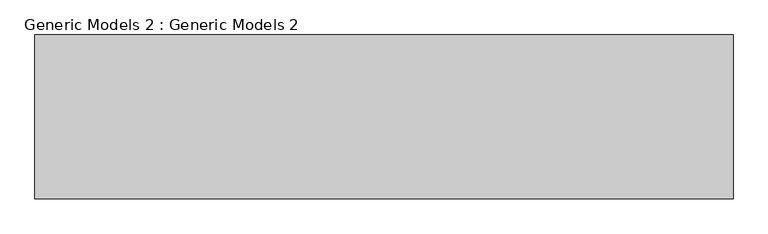
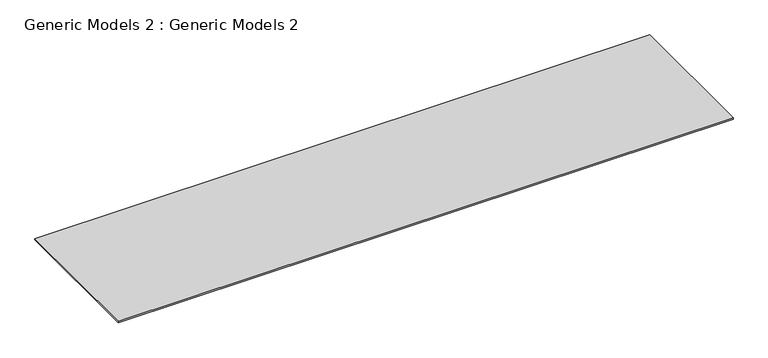
"""IFC4 building model written with IfcOpenShell, lengths in millimetres: proxy geometry, Generic Models 2 : Generic Models 2."""

from ifc_helpers import new_model, si_unit, origin, origin_with_axes, place, context, project, spatial, polyline, outline, extrude, source, transform, mapped, element, save


def generic_models_2_generic_models_2_6ec805a2(model_context):
    return source(origin(), model_context, "Body", "SweptSolid", [
        extrude(outline(polyline([(21097.8872949, 22221.9257991), (-14284.3889776, 22221.9257991), (-14284.3889776, 30521.0482451), (21097.8872949, 30521.0482451), (21097.8872949, 22221.9257991)])), origin_with_axes(), (0.0, 0.0, 1.0), 85.9299213),
    ])


if __name__ == "__main__":
    model = new_model("IFC4")
    model_context = context("Model", 3, world=origin())
    ifc_project = project(units=[si_unit("LENGTHUNIT", "METRE", prefix="MILLI")], contexts=[model_context])
    site = spatial("IfcSite", under=ifc_project)
    building = spatial("IfcBuilding", under=site)
    placement = place(None, origin())
    generic_models_2_generic_models_2_shape = generic_models_2_generic_models_2_6ec805a2(model_context)
    element("IfcBuildingElementProxy", 1, Name="Generic Models 2 : Generic Models 2", ObjectType="Generic Models 2 : Generic Models 2", at=placement, inside=building, context=model_context, shape_type="MappedRepresentation", body=[
        mapped(generic_models_2_generic_models_2_shape, transform((0.0, 0.0, 0.0), x_axis=(1.0, 0.0, 0.0), y_axis=(0.0, 1.0, 0.0), z_axis=(0.0, 0.0, 1.0))),
    ])
    save(model, "model.ifc")
